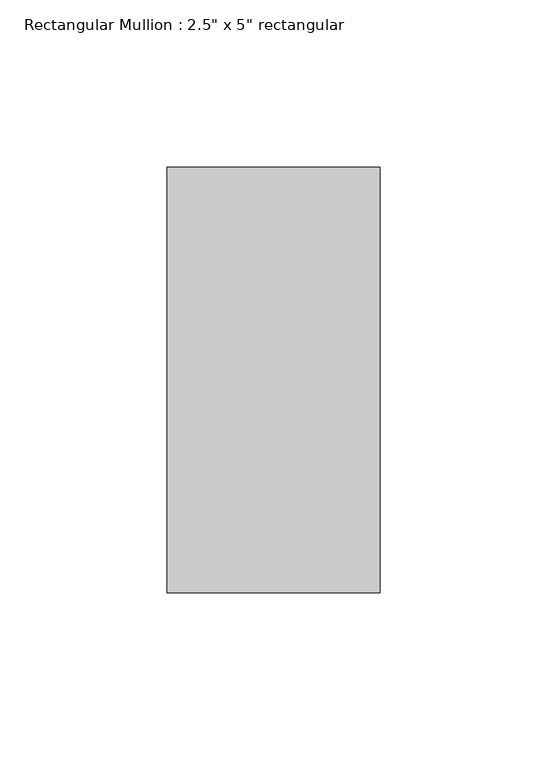
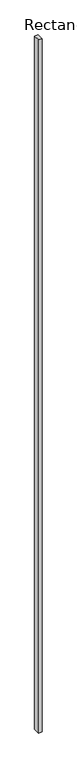
"""IFC4 building model written with IfcOpenShell, lengths in millimetres: member geometry."""

from ifc_helpers import new_model, si_unit, frame, origin, place, context, project, spatial, polyline, outline, extrude, source, transform, mapped, element, save


def member_e7df1716(model_context):
    return source(origin(), model_context, "Body", "SweptSolid", [
        extrude(outline(polyline([(0.0, 63.5), (0.0, -63.5), (-63.5, -63.5), (-63.5, 63.5), (0.0, 63.5)])), frame((0.0, 0.0, -13650.77075), z_axis=(0.0, 0.0, 1.0), x_axis=(1.0, 0.0, 0.0)), (0.0, 0.0, 1.0), 13650.77075),
    ])


if __name__ == "__main__":
    model = new_model("IFC4")
    model_context = context("Model", 3, world=origin())
    ifc_project = project(units=[si_unit("LENGTHUNIT", "METRE", prefix="MILLI")], contexts=[model_context])
    site = spatial("IfcSite", under=ifc_project)
    building = spatial("IfcBuilding", under=site)
    placement = place(None, origin())
    member_shape = member_e7df1716(model_context)
    element("IfcMember", 1, ObjectType="Rectangular Mullion : 2.5\" x 5\" rectangular", at=placement, inside=building, context=model_context, shape_type="MappedRepresentation", body=[
        mapped(member_shape, transform((0.0, 0.0, 0.0), x_axis=(1.0, 0.0, 0.0), y_axis=(0.0, 1.0, 0.0), z_axis=(0.0, 0.0, 1.0))),
    ])
    save(model, "model.ifc")

# Revit data of these elements
# Type "Rectangular Mullion : 2.5\" x 5\" rectangular"
#   built-in parameter 1007304 = 0.416667 (stored number, unit not read)
#   built-in parameter 1007301 = 0.104167 (stored number, unit not read)
#   built-in parameter 1007300 = 0.104167 (stored number, unit not read)
# Element 1 (IfcMember, "Rectangular Mullion : 2.5\" x 5\" rectangular")
#   Materials on its faces: "Aluminum"
# Materials
#   "Aluminum": class "Metal", colour RGB 247 247 247, transparency 0, Description = "Aluminum 6061", Cost = 0
